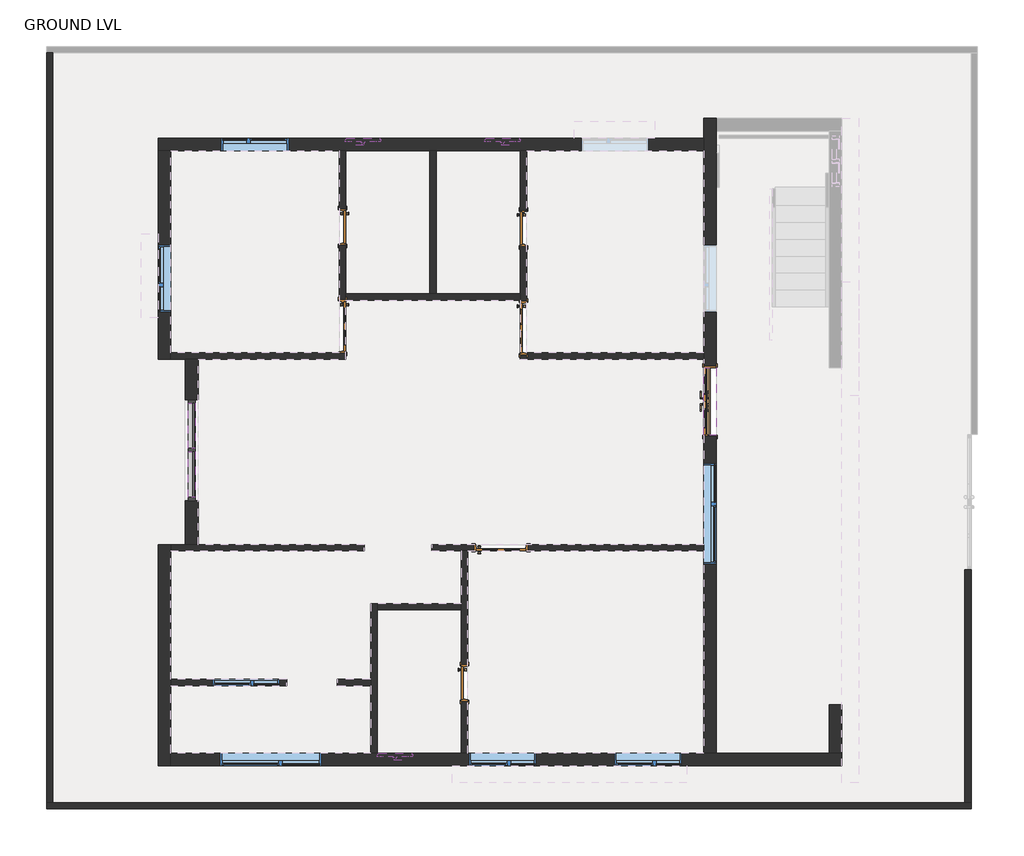
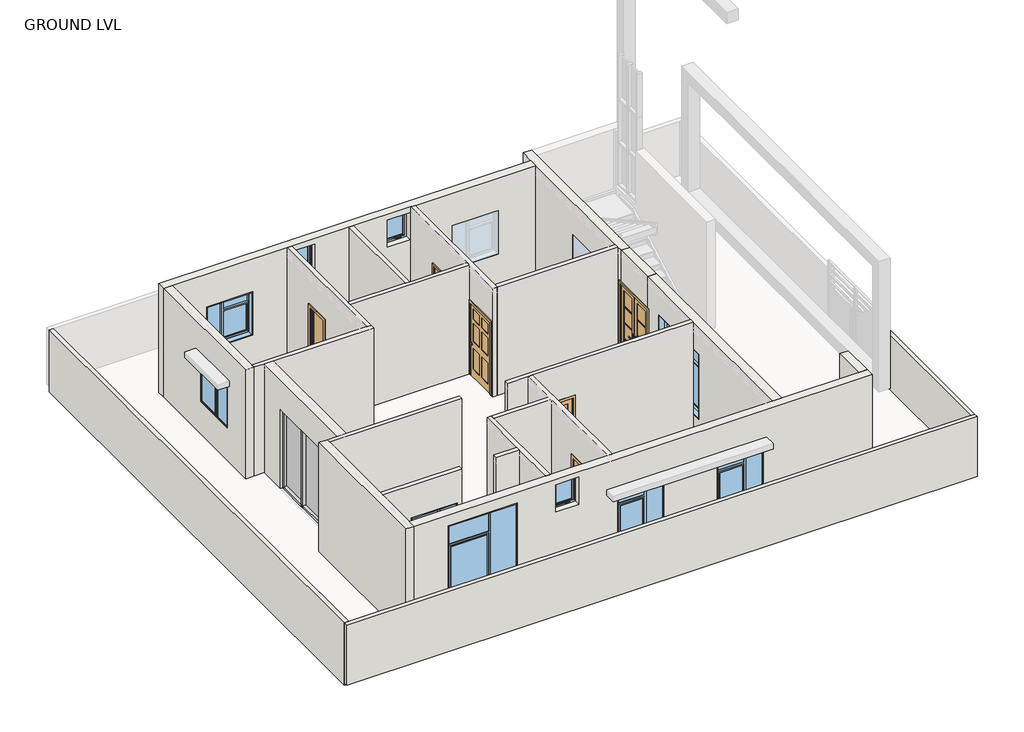
# One storey, part 1 of 2: 25 walls, 10 windows, 7 doors, 7 members, 2 plates.
"""IFC4 building model written with IfcOpenShell, lengths in millimetres."""

from ifc_helpers import new_model, si_unit, frame, origin, origin_with_axes, place, context, project, spatial, polyline, outline, extrude, faceted_brep, transform, mapped, element, save
from components import door_exterior_double_full_glass_wood_clad_double_main_door_4_3788f36b, door_92bad2d9, door_a4da38fb, door_0e119d28, door_525aa856, member_c17f1be2, member_acd63386, member_c841a703, system_panel_glazed_ef5431d1, window_610_x_762_5077743b, window_610_x_762_22856471, window_casement_double_sidelight_window_4_x_4_2a492e8f, window_casement_double_sidelight_window_4_x_4_ae1e99d1, window_casement_double_sidelight_window_6_x_6_6a7c62ef

model = new_model("IFC4")

# Units and contexts
model_context = context("Model", 3, world=origin())
ifc_project = project(units=[si_unit("LENGTHUNIT", "METRE", prefix="MILLI")], contexts=[model_context])

# Site, building, storey
site = spatial("IfcSite", under=ifc_project)
building = spatial("IfcBuilding", under=site)
storey = spatial("IfcBuildingStorey", under=building, Name="GROUND LVL", Elevation=0.0)

# Doors
placement = place(None, origin())
door_exterior_double_full_glass_wood_clad_double_main_door_4_shape = door_exterior_double_full_glass_wood_clad_double_main_door_4_3788f36b(model_context)
element("IfcDoor", 1, ObjectType="Door-Exterior-Double-Full Glass-Wood_Clad : double main door 4' x 7'", at=placement, inside=storey, context=model_context, shape_type="MappedRepresentation", body=[
    mapped(door_exterior_double_full_glass_wood_clad_double_main_door_4_shape, transform((-4646.5406154, 1972.1500875, -25.4), x_axis=(0.0, 1.0, 0.0), y_axis=(-1.0, 0.0, 0.0), z_axis=(0.0, 0.0, 1.0))),
])
door_shape = door_92bad2d9(model_context)
element("IfcDoor", 2, ObjectType="Door-Interior-Single-6_Panel-Wood : 36\" x 80\"", at=placement, inside=storey, context=model_context, shape_type="MappedRepresentation", body=[
    mapped(door_shape, transform((-11288.6406154, 3324.7000875, 0.0), x_axis=(0.0, -1.0, 0.0), y_axis=(1.0, 0.0, 0.0), z_axis=(0.0, 0.0, 1.0))),
])
door_2_shape = door_a4da38fb(model_context)
element("IfcDoor", 3, ObjectType="Door-Interior-Single-6_Panel-Wood : 36\" x 80\"", at=placement, inside=storey, context=model_context, shape_type="MappedRepresentation", body=[
    mapped(door_2_shape, transform((-8018.3906154, 3299.3000875, 0.0), x_axis=(0.0, -1.0, 0.0), y_axis=(1.0, 0.0, 0.0), z_axis=(0.0, 0.0, 1.0))),
])
element("IfcDoor", 4, ObjectType="Door-Interior-Single-6_Panel-Wood : 36\" x 80\"", at=placement, inside=storey, context=model_context, shape_type="MappedRepresentation", body=[
    mapped(door_2_shape, transform((-8421.6156154, -678.9749125, 0.0), x_axis=(1.0, 0.0, 0.0), y_axis=(0.0, 1.0, 0.0), z_axis=(0.0, 0.0, 1.0))),
])
door_3_shape = door_0e119d28(model_context)
element("IfcDoor", 5, ObjectType="Door-Interior-Single-Flush_Panel-Wood : 24\" x 80\"", at=placement, inside=storey, context=model_context, shape_type="MappedRepresentation", body=[
    mapped(door_3_shape, transform((-11288.6406154, 5128.1000875, 0.0), x_axis=(0.0, -1.0, 0.0), y_axis=(1.0, 0.0, 0.0), z_axis=(0.0, 0.0, 1.0))),
])
door_4_shape = door_525aa856(model_context)
element("IfcDoor", 6, ObjectType="Door-Interior-Single-Flush_Panel-Wood : 24\" x 80\"", at=placement, inside=storey, context=model_context, shape_type="MappedRepresentation", body=[
    mapped(door_4_shape, transform((-8018.3906154, 5102.7000875, 0.0), x_axis=(0.0, -1.0, 0.0), y_axis=(1.0, 0.0, 0.0), z_axis=(0.0, 0.0, 1.0))),
])
element("IfcDoor", 7, ObjectType="Door-Interior-Single-Flush_Panel-Wood : 24\" x 80\"", at=placement, inside=storey, context=model_context, shape_type="MappedRepresentation", body=[
    mapped(door_4_shape, transform((-9085.1906154, -3123.7249125, 0.0), x_axis=(0.0, -1.0, 0.0), y_axis=(1.0, 0.0, 0.0), z_axis=(0.0, 0.0, 1.0))),
])

# Members
member_shape = member_c17f1be2(model_context)
element("IfcMember", 8, ObjectType="Rectangular Mullion : 2.5\" x 5\" rectangular", at=placement, inside=storey, context=model_context, shape_type="MappedRepresentation", body=[
    mapped(member_shape, transform((-14015.9656154, 238.6000875, 2214.7649104), x_axis=(0.0, 0.0, 1.0), y_axis=(-1.0, 0.0, 0.0), z_axis=(0.0, -1.0, 0.0))),
])
element("IfcMember", 9, ObjectType="Rectangular Mullion : 2.5\" x 5\" rectangular", at=placement, inside=storey, context=model_context, shape_type="MappedRepresentation", body=[
    mapped(member_shape, transform((-14015.9656154, 1121.2500875, 2214.7649104), x_axis=(0.0, 0.0, 1.0), y_axis=(-1.0, 0.0, 0.0), z_axis=(0.0, -1.0, 0.0))),
])
element("IfcMember", 10, ObjectType="Rectangular Mullion : 2.5\" x 5\" rectangular", at=placement, inside=storey, context=model_context, shape_type="MappedRepresentation", body=[
    mapped(member_shape, transform((-14015.9656154, 1940.4000875, 0.0), x_axis=(0.0, 0.0, -1.0), y_axis=(-1.0, 0.0, 0.0), z_axis=(0.0, 1.0, 0.0))),
])
element("IfcMember", 11, ObjectType="Rectangular Mullion : 2.5\" x 5\" rectangular", at=placement, inside=storey, context=model_context, shape_type="MappedRepresentation", body=[
    mapped(member_shape, transform((-14015.9656154, 1057.7500875, 0.0), x_axis=(0.0, 0.0, -1.0), y_axis=(-1.0, 0.0, 0.0), z_axis=(0.0, 1.0, 0.0))),
])
member_2_shape = member_acd63386(model_context)
element("IfcMember", 12, ObjectType="Rectangular Mullion : 2.5\" x 5\" rectangular", at=placement, inside=storey, context=model_context, shape_type="MappedRepresentation", body=[
    mapped(member_2_shape, transform((-14015.9656154, 1089.5000875, 0.0), x_axis=(0.0, -1.0, 0.0), y_axis=(-1.0, 0.0, 0.0), z_axis=(0.0, 0.0, -1.0))),
])
member_3_shape = member_c841a703(model_context)
element("IfcMember", 13, ObjectType="Rectangular Mullion : 2.5\" x 5\" rectangular", at=placement, inside=storey, context=model_context, shape_type="MappedRepresentation", body=[
    mapped(member_3_shape, transform((-14015.9656154, 175.1000875, 0.0), x_axis=(0.0, -1.0, 0.0), y_axis=(-1.0, 0.0, 0.0), z_axis=(0.0, 0.0, -1.0))),
])
element("IfcMember", 14, ObjectType="Rectangular Mullion : 2.5\" x 5\" rectangular", at=placement, inside=storey, context=model_context, shape_type="MappedRepresentation", body=[
    mapped(member_3_shape, transform((-14015.9656154, 2003.9000875, 2214.7649104), x_axis=(0.0, 1.0, 0.0), y_axis=(-1.0, 0.0, 0.0), z_axis=(0.0, 0.0, 1.0))),
])

# Plates
system_panel_glazed_shape = system_panel_glazed_ef5431d1(model_context)
element("IfcPlate", 15, ObjectType="System Panel : Glazed", at=placement, inside=storey, context=model_context, shape_type="MappedRepresentation", body=[
    mapped(system_panel_glazed_shape, transform((-14015.9656154, 1530.8250875, 63.5), x_axis=(0.0, -1.0, 0.0), y_axis=(1.0, 0.0, 0.0), z_axis=(0.0, 0.0, 1.0))),
])
element("IfcPlate", 16, ObjectType="System Panel : Glazed", at=placement, inside=storey, context=model_context, shape_type="MappedRepresentation", body=[
    mapped(system_panel_glazed_shape, transform((-14015.9656154, 648.1750875, 63.5), x_axis=(0.0, -1.0, 0.0), y_axis=(1.0, 0.0, 0.0), z_axis=(0.0, 0.0, 1.0))),
])

# Walls
element("IfcWall", 17, at=placement, inside=storey, context=model_context, shape_type="Brep", body=[
    faceted_brep([(-4757.6656154, 6734.6500875, 0.0), (-14625.5656154, 6734.6500875, 0.0), (-14625.5656154, 6734.6500875, 3048.0), (-4757.6656154, 6734.6500875, 3048.0), (-10612.3656154, 6734.6500875, 2133.6), (-10612.3656154, 6734.6500875, 2895.6), (-11221.9656154, 6734.6500875, 2895.6), (-11221.9656154, 6734.6500875, 2133.6), (-8701.0156154, 6734.6500875, 2895.6), (-8701.0156154, 6734.6500875, 2133.6), (-8091.4156154, 6734.6500875, 2133.6), (-8091.4156154, 6734.6500875, 2895.6), (-5748.2656154, 6734.6500875, 2133.6), (-6967.4656154, 6734.6500875, 2133.6), (-6967.4656154, 6734.6500875, 914.4), (-5748.2656154, 6734.6500875, 914.4), (-12263.3656154, 6734.6500875, 2133.6), (-13482.5656154, 6734.6500875, 2133.6), (-13482.5656154, 6734.6500875, 914.4), (-12263.3656154, 6734.6500875, 914.4), (-4757.6656154, 6506.0500875, 0.0), (-4757.6656154, 6506.0500875, 3048.0), (-7958.0656154, 6506.0500875, 3048.0), (-8072.3656154, 6506.0500875, 3048.0), (-9596.3656154, 6506.0500875, 3048.0), (-9710.6656154, 6506.0500875, 3048.0), (-11234.6656154, 6506.0500875, 3048.0), (-11348.9656154, 6506.0500875, 3048.0), (-14396.9656154, 6506.0500875, 3048.0), (-14625.5656154, 6506.0500875, 3048.0), (-14625.5656154, 6506.0500875, 0.0), (-14396.9656154, 6506.0500875, 0.0), (-11348.9656154, 6506.0500875, 0.0), (-11234.6656154, 6506.0500875, 0.0), (-9710.6656154, 6506.0500875, 0.0), (-9596.3656154, 6506.0500875, 0.0), (-8072.3656154, 6506.0500875, 0.0), (-7958.0656154, 6506.0500875, 0.0), (-10612.3656154, 6506.0500875, 2895.6), (-10612.3656154, 6506.0500875, 2133.6), (-11221.9656154, 6506.0500875, 2133.6), (-11221.9656154, 6506.0500875, 2895.6), (-8701.0156154, 6506.0500875, 2133.6), (-8701.0156154, 6506.0500875, 2895.6), (-8091.4156154, 6506.0500875, 2895.6), (-8091.4156154, 6506.0500875, 2133.6), (-5748.2656154, 6506.0500875, 2133.6), (-5748.2656154, 6506.0500875, 914.4), (-6967.4656154, 6506.0500875, 914.4), (-6967.4656154, 6506.0500875, 2133.6), (-12263.3656154, 6506.0500875, 2133.6), (-12263.3656154, 6506.0500875, 914.4), (-13482.5656154, 6506.0500875, 914.4), (-13482.5656154, 6506.0500875, 2133.6)], [[[0, 1, 2, 3], [4, 5, 6, 7], [8, 9, 10, 11], [12, 13, 14, 15], [16, 17, 18, 19]], [[20, 21, 22, 23, 24, 25, 26, 27, 28, 29, 30, 31, 32, 33, 34, 35, 36, 37], [38, 39, 40, 41], [42, 43, 44, 45], [46, 47, 48, 49], [50, 51, 52, 53]], [[1, 0, 20, 37, 36, 35, 34, 33, 32, 31, 30]], [[3, 2, 29, 28, 27, 26, 25, 24, 23, 22, 21]], [[2, 1, 30, 29]], [[39, 38, 5, 4]], [[4, 7, 40, 39]], [[7, 6, 41, 40]], [[38, 41, 6, 5]], [[42, 9, 8, 43]], [[9, 42, 45, 10]], [[10, 45, 44, 11]], [[43, 8, 11, 44]], [[47, 46, 12, 15]], [[48, 47, 15, 14]], [[49, 48, 14, 13]], [[46, 49, 13, 12]], [[51, 50, 16, 19]], [[52, 51, 19, 18]], [[53, 52, 18, 17]], [[50, 53, 17, 16]], [[0, 3, 21, 20]]]),
])
element("IfcWall", 18, at=placement, inside=storey, context=model_context, shape_type="Brep", body=[
    faceted_brep([(-14625.5656154, 6506.0500875, 0.0), (-14625.5656154, 2734.1500875, 0.0), (-14625.5656154, 2734.1500875, 3048.0), (-14625.5656154, 6506.0500875, 3048.0), (-14625.5656154, 4803.1295492, 2133.6), (-14625.5656154, 3583.9295492, 2133.6), (-14625.5656154, 3583.9295492, 914.4), (-14625.5656154, 4803.1295492, 914.4), (-14396.9656154, 6506.0500875, 0.0), (-14396.9656154, 6506.0500875, 3048.0), (-14396.9656154, 2848.4500875, 3048.0), (-14396.9656154, 2734.1500875, 3048.0), (-14396.9656154, 2734.1500875, 0.0), (-14396.9656154, 2848.4500875, 0.0), (-14396.9656154, 4803.1295492, 2133.6), (-14396.9656154, 4803.1295492, 914.4), (-14396.9656154, 3583.9295492, 914.4), (-14396.9656154, 3583.9295492, 2133.6)], [[[0, 1, 2, 3], [4, 5, 6, 7]], [[8, 9, 10, 11, 12, 13], [14, 15, 16, 17]], [[1, 0, 8, 13, 12]], [[3, 2, 11, 10, 9]], [[0, 3, 9, 8]], [[2, 1, 12, 11]], [[15, 14, 4, 7]], [[16, 15, 7, 6]], [[17, 16, 6, 5]], [[14, 17, 5, 4]]]),
])
element("IfcWall", 19, at=placement, inside=storey, context=model_context, shape_type="Brep", body=[
    faceted_brep([(-14625.5656154, -618.6499125, 0.0), (-14625.5656154, -4619.1499125, 0.0), (-14625.5656154, -4619.1499125, 3048.0), (-14625.5656154, -618.6499125, 3048.0), (-14396.9656154, -618.6499125, 0.0), (-14396.9656154, -618.6499125, 3048.0), (-14396.9656154, -732.9499125, 3048.0), (-14396.9656154, -3057.0499125, 3048.0), (-14396.9656154, -3171.3499125, 3048.0), (-14396.9656154, -4390.5499125, 3048.0), (-14396.9656154, -4619.1499125, 3048.0), (-14396.9656154, -4619.1499125, 0.0), (-14396.9656154, -4390.5499125, 0.0), (-14396.9656154, -3171.3499125, 0.0), (-14396.9656154, -3057.0499125, 0.0), (-14396.9656154, -732.9499125, 0.0)], [[[0, 1, 2, 3]], [[4, 5, 6, 7, 8, 9, 10, 11, 12, 13, 14, 15]], [[1, 0, 4, 15, 14, 13, 12, 11]], [[3, 2, 10, 9, 8, 7, 6, 5]], [[2, 1, 11, 10]], [[0, 3, 5, 4]]]),
])
element("IfcWall", 20, at=placement, inside=storey, context=model_context, shape_type="Brep", body=[
    faceted_brep([(-14396.9656154, -4619.1499125, 0.0), (-2255.7656154, -4619.1499125, 0.0), (-2255.7656154, -4619.1499125, 3048.0), (-14396.9656154, -4619.1499125, 3048.0), (-10644.1156154, -4619.1499125, 2133.6), (-10644.1156154, -4619.1499125, 2895.6), (-10034.5156154, -4619.1499125, 2895.6), (-10034.5156154, -4619.1499125, 2133.6), (-9005.8156154, -4619.1499125, 2133.6), (-7786.6156154, -4619.1499125, 2133.6), (-7786.6156154, -4619.1499125, 914.4), (-9005.8156154, -4619.1499125, 914.4), (-6370.5656154, -4619.1499125, 2133.6), (-5151.3656154, -4619.1499125, 2133.6), (-5151.3656154, -4619.1499125, 914.4), (-6370.5656154, -4619.1499125, 914.4), (-13501.6156154, -4619.1499125, 2743.2), (-11672.8156154, -4619.1499125, 2743.2), (-11672.8156154, -4619.1499125, 914.4), (-13501.6156154, -4619.1499125, 914.4), (-14396.9656154, -4390.5499125, 0.0), (-14396.9656154, -4390.5499125, 3048.0), (-10777.4656154, -4390.5499125, 3048.0), (-10663.1656154, -4390.5499125, 3048.0), (-9139.1656154, -4390.5499125, 3048.0), (-9024.8656154, -4390.5499125, 3048.0), (-4757.6656154, -4390.5499125, 3048.0), (-4529.0656154, -4390.5499125, 3048.0), (-2484.3656154, -4390.5499125, 3048.0), (-2255.7656154, -4390.5499125, 3048.0), (-2255.7656154, -4390.5499125, 0.0), (-2484.3656154, -4390.5499125, 0.0), (-4529.0656154, -4390.5499125, 0.0), (-4757.6656154, -4390.5499125, 0.0), (-9024.8656154, -4390.5499125, 0.0), (-9139.1656154, -4390.5499125, 0.0), (-10663.1656154, -4390.5499125, 0.0), (-10777.4656154, -4390.5499125, 0.0), (-10644.1156154, -4390.5499125, 2895.6), (-10644.1156154, -4390.5499125, 2133.6), (-10034.5156154, -4390.5499125, 2133.6), (-10034.5156154, -4390.5499125, 2895.6), (-9005.8156154, -4390.5499125, 2133.6), (-9005.8156154, -4390.5499125, 914.4), (-7786.6156154, -4390.5499125, 914.4), (-7786.6156154, -4390.5499125, 2133.6), (-6370.5656154, -4390.5499125, 2133.6), (-6370.5656154, -4390.5499125, 914.4), (-5151.3656154, -4390.5499125, 914.4), (-5151.3656154, -4390.5499125, 2133.6), (-13501.6156154, -4390.5499125, 2743.2), (-13501.6156154, -4390.5499125, 914.4), (-11672.8156154, -4390.5499125, 914.4), (-11672.8156154, -4390.5499125, 2743.2)], [[[0, 1, 2, 3], [4, 5, 6, 7], [8, 9, 10, 11], [12, 13, 14, 15], [16, 17, 18, 19]], [[20, 21, 22, 23, 24, 25, 26, 27, 28, 29, 30, 31, 32, 33, 34, 35, 36, 37], [38, 39, 40, 41], [42, 43, 44, 45], [46, 47, 48, 49], [50, 51, 52, 53]], [[1, 0, 20, 37, 36, 35, 34, 33, 32, 31, 30]], [[3, 2, 29, 28, 27, 26, 25, 24, 23, 22, 21]], [[0, 3, 21, 20]], [[4, 39, 38, 5]], [[39, 4, 7, 40]], [[40, 7, 6, 41]], [[5, 38, 41, 6]], [[43, 42, 8, 11]], [[44, 43, 11, 10]], [[45, 44, 10, 9]], [[42, 45, 9, 8]], [[47, 46, 12, 15]], [[48, 47, 15, 14]], [[49, 48, 14, 13]], [[46, 49, 13, 12]], [[51, 50, 16, 19]], [[52, 51, 19, 18]], [[53, 52, 18, 17]], [[50, 53, 17, 16]], [[2, 1, 30, 29]]]),
])
element("IfcWall", 21, at=placement, inside=storey, context=model_context, shape_type="Brep", body=[
    faceted_brep([(-4529.0656154, 1362.5500875, 3048.0), (-4529.0656154, -4390.5499125, 3048.0), (-4529.0656154, -4390.5499125, 0.0), (-4529.0656154, 1337.1500875, 0.0), (-4529.0656154, 1337.1500875, 2133.6), (-4529.0656154, 1362.5500875, 2133.6), (-4529.0656154, -976.6434232, 2286.0), (-4529.0656154, 852.1565768, 2286.0), (-4529.0656154, 852.1565768, 457.2), (-4529.0656154, -976.6434232, 457.2), (-4757.6656154, -4390.5499125, 3048.0), (-4757.6656154, -732.9499125, 3048.0), (-4757.6656154, -618.6499125, 3048.0), (-4757.6656154, 1362.5500875, 3048.0), (-4757.6656154, 1362.5500875, 2133.6), (-4757.6656154, 1337.1500875, 2133.6), (-4757.6656154, 1337.1500875, 0.0), (-4757.6656154, -618.6499125, 0.0), (-4757.6656154, -732.9499125, 0.0), (-4757.6656154, -4390.5499125, 0.0), (-4757.6656154, -976.6434232, 2286.0), (-4757.6656154, -976.6434232, 457.2), (-4757.6656154, 852.1565768, 457.2), (-4757.6656154, 852.1565768, 2286.0)], [[[0, 1, 2, 3, 4, 5], [6, 7, 8, 9]], [[10, 11, 12, 13, 14, 15, 16, 17, 18, 19], [20, 21, 22, 23]], [[2, 19, 18, 17, 16, 3]], [[13, 0, 5, 14]], [[1, 0, 13, 12, 11, 10]], [[2, 1, 10, 19]], [[4, 15, 14, 5]], [[15, 4, 3, 16]], [[21, 20, 6, 9]], [[22, 21, 9, 8]], [[23, 22, 8, 7]], [[20, 23, 7, 6]]]),
])
element("IfcWall", 22, at=placement, inside=storey, context=model_context, shape_type="Brep", body=[
    faceted_brep([(-4529.0656154, 7090.2500875, 3048.0), (-4529.0656154, 6861.6500875, 3048.0), (-4529.0656154, 2581.7500875, 3048.0), (-4529.0656154, 2581.7500875, 2133.6), (-4529.0656154, 2607.1500875, 2133.6), (-4529.0656154, 2607.1500875, 0.0), (-4529.0656154, 6861.6500875, 0.0), (-4529.0656154, 7090.2500875, 0.0), (-4529.0656154, 4803.1295492, 2133.6), (-4529.0656154, 4803.1295492, 914.4), (-4529.0656154, 3583.9295492, 914.4), (-4529.0656154, 3583.9295492, 2133.6), (-4757.6656154, 2581.7500875, 3048.0), (-4757.6656154, 2734.1500875, 3048.0), (-4757.6656154, 2848.4500875, 3048.0), (-4757.6656154, 6506.0500875, 3048.0), (-4757.6656154, 6734.6500875, 3048.0), (-4757.6656154, 7090.2500875, 3048.0), (-4757.6656154, 7090.2500875, 0.0), (-4757.6656154, 6734.6500875, 0.0), (-4757.6656154, 6506.0500875, 0.0), (-4757.6656154, 2848.4500875, 0.0), (-4757.6656154, 2734.1500875, 0.0), (-4757.6656154, 2607.1500875, 0.0), (-4757.6656154, 2607.1500875, 2133.6), (-4757.6656154, 2581.7500875, 2133.6), (-4757.6656154, 4803.1295492, 2133.6), (-4757.6656154, 3583.9295492, 2133.6), (-4757.6656154, 3583.9295492, 914.4), (-4757.6656154, 4803.1295492, 914.4)], [[[0, 1, 2, 3, 4, 5, 6, 7], [8, 9, 10, 11]], [[12, 13, 14, 15, 16, 17, 18, 19, 20, 21, 22, 23, 24, 25], [26, 27, 28, 29]], [[18, 7, 6, 5, 23, 22, 21, 20, 19]], [[2, 1, 0, 17, 16, 15, 14, 13, 12]], [[2, 12, 25, 3]], [[4, 24, 23, 5]], [[24, 4, 3, 25]], [[9, 8, 26, 29]], [[10, 9, 29, 28]], [[11, 10, 28, 27]], [[8, 11, 27, 26]], [[0, 7, 18, 17]]]),
])
element("IfcWall", 23, at=placement, inside=storey, context=model_context, shape_type="Brep", body=[
    faceted_brep([(-14396.9656154, -732.9499125, 0.0), (-10895.4913348, -732.9499125, 0.0), (-10895.4913348, -732.9499125, 3048.0), (-14396.9656154, -732.9499125, 3048.0), (-14396.9656154, -618.6499125, 0.0), (-14396.9656154, -618.6499125, 3048.0), (-14130.2656154, -618.6499125, 3048.0), (-13901.6656154, -618.6499125, 3048.0), (-10895.4913348, -618.6499125, 3048.0), (-10895.4913348, -618.6499125, 0.0), (-13901.6656154, -618.6499125, 0.0), (-14130.2656154, -618.6499125, 0.0)], [[[0, 1, 2, 3]], [[4, 5, 6, 7, 8, 9, 10, 11]], [[1, 0, 4, 11, 10, 9]], [[2, 1, 9, 8]], [[3, 2, 8, 7, 6, 5]], [[0, 3, 5, 4]]]),
])
element("IfcWall", 24, at=placement, inside=storey, context=model_context, shape_type="SweptSolid", body=[
    extrude(outline(polyline([(0.0, -14396.9656154), (0.0, -12301.4656154), (3048.0, -12301.4656154), (3048.0, -14396.9656154), (0.0, -14396.9656154)]), holes=[polyline([(2133.6, -13647.6656154), (2133.6, -12428.4656154), (914.4, -12428.4656154), (914.4, -13647.6656154), (2133.6, -13647.6656154)])]), frame((0.0, -3171.3499125, 0.0), z_axis=(0.0, 1.0, 0.0), x_axis=(0.0, 0.0, 1.0)), (0.0, 0.0, 1.0), 114.3),
])
element("IfcWall", 25, at=placement, inside=storey, context=model_context, shape_type="SweptSolid", body=[
    extrude(outline(polyline([(-11387.0656154, -3057.0499125), (-10777.4656154, -3057.0499125), (-10777.4656154, -3171.3499125), (-11387.0656154, -3171.3499125), (-11387.0656154, -3057.0499125)])), origin_with_axes(), (0.0, 0.0, 1.0), 3048.0),
])
element("IfcWall", 26, at=placement, inside=storey, context=model_context, shape_type="Brep", body=[
    faceted_brep([(-10663.1656154, -4390.5499125, 0.0), (-10663.1656154, -1799.7499125, 0.0), (-10663.1656154, -1685.4499125, 0.0), (-10663.1656154, -1685.4499125, 3048.0), (-10663.1656154, -1799.7499125, 3048.0), (-10663.1656154, -4390.5499125, 3048.0), (-10777.4656154, -4390.5499125, 0.0), (-10777.4656154, -4390.5499125, 3048.0), (-10777.4656154, -3171.3499125, 3048.0), (-10777.4656154, -3057.0499125, 3048.0), (-10777.4656154, -1685.4499125, 3048.0), (-10777.4656154, -1685.4499125, 0.0), (-10777.4656154, -3057.0499125, 0.0), (-10777.4656154, -3171.3499125, 0.0)], [[[0, 1, 2, 3, 4, 5]], [[6, 7, 8, 9, 10, 11, 12, 13]], [[2, 1, 0, 6, 13, 12, 11]], [[5, 4, 3, 10, 9, 8, 7]], [[0, 5, 7, 6]], [[3, 2, 11, 10]]]),
])
element("IfcWall", 27, at=placement, inside=storey, context=model_context, shape_type="SweptSolid", body=[
    extrude(outline(polyline([(-9139.1656154, -1799.7499125), (-10663.1656154, -1799.7499125), (-10663.1656154, -1685.4499125), (-9139.1656154, -1685.4499125), (-9139.1656154, -1799.7499125)])), origin_with_axes(), (0.0, 0.0, 1.0), 3048.0),
])
element("IfcWall", 28, at=placement, inside=storey, context=model_context, shape_type="Brep", body=[
    faceted_brep([(-9024.8656154, -732.9499125, 3048.0), (-9024.8656154, -4390.5499125, 3048.0), (-9024.8656154, -4390.5499125, 0.0), (-9024.8656154, -3453.9249125, 0.0), (-9024.8656154, -3453.9249125, 2057.4), (-9024.8656154, -2793.5249125, 2057.4), (-9024.8656154, -2793.5249125, 0.0), (-9024.8656154, -732.9499125, 0.0), (-9139.1656154, -4390.5499125, 3048.0), (-9139.1656154, -1799.7499125, 3048.0), (-9139.1656154, -1685.4499125, 3048.0), (-9139.1656154, -732.9499125, 3048.0), (-9139.1656154, -732.9499125, 0.0), (-9139.1656154, -1685.4499125, 0.0), (-9139.1656154, -1799.7499125, 0.0), (-9139.1656154, -2793.5249125, 0.0), (-9139.1656154, -2793.5249125, 2057.4), (-9139.1656154, -3453.9249125, 2057.4), (-9139.1656154, -3453.9249125, 0.0), (-9139.1656154, -4390.5499125, 0.0)], [[[0, 1, 2, 3, 4, 5, 6, 7]], [[8, 9, 10, 11, 12, 13, 14, 15, 16, 17, 18, 19]], [[12, 7, 6, 15, 14, 13]], [[2, 19, 18, 3]], [[1, 0, 11, 10, 9, 8]], [[0, 7, 12, 11]], [[2, 1, 8, 19]], [[17, 4, 3, 18]], [[4, 17, 16, 5]], [[5, 16, 15, 6]]]),
])
element("IfcWall", 29, at=placement, inside=storey, context=model_context, shape_type="Brep", body=[
    faceted_brep([(-8072.3656154, 2734.1500875, 3048.0), (-8072.3656154, 3800.9500875, 3048.0), (-8072.3656154, 3915.2500875, 3048.0), (-8072.3656154, 6506.0500875, 3048.0), (-8072.3656154, 6506.0500875, 0.0), (-8072.3656154, 5432.9000875, 0.0), (-8072.3656154, 5432.9000875, 2057.4), (-8072.3656154, 4772.5000875, 2057.4), (-8072.3656154, 4772.5000875, 0.0), (-8072.3656154, 3915.2500875, 0.0), (-8072.3656154, 3800.9500875, 0.0), (-8072.3656154, 3781.9000875, 0.0), (-8072.3656154, 3781.9000875, 2057.4), (-8072.3656154, 2816.7000875, 2057.4), (-8072.3656154, 2816.7000875, 0.0), (-8072.3656154, 2734.1500875, 0.0), (-7958.0656154, 6506.0500875, 3048.0), (-7958.0656154, 2848.4500875, 3048.0), (-7958.0656154, 2734.1500875, 3048.0), (-7958.0656154, 2734.1500875, 0.0), (-7958.0656154, 2816.7000875, 0.0), (-7958.0656154, 2816.7000875, 2057.4), (-7958.0656154, 3781.9000875, 2057.4), (-7958.0656154, 3781.9000875, 0.0), (-7958.0656154, 4772.5000875, 0.0), (-7958.0656154, 4772.5000875, 2057.4), (-7958.0656154, 5432.9000875, 2057.4), (-7958.0656154, 5432.9000875, 0.0), (-7958.0656154, 6506.0500875, 0.0)], [[[0, 1, 2, 3, 4, 5, 6, 7, 8, 9, 10, 11, 12, 13, 14, 15]], [[16, 17, 18, 19, 20, 21, 22, 23, 24, 25, 26, 27, 28]], [[4, 28, 27, 5]], [[19, 15, 14, 20]], [[23, 11, 10, 9, 8, 24]], [[3, 2, 1, 0, 18, 17, 16]], [[4, 3, 16, 28]], [[0, 15, 19, 18]], [[14, 13, 21, 20]], [[13, 12, 22, 21]], [[12, 11, 23, 22]], [[7, 25, 24, 8]], [[25, 7, 6, 26]], [[26, 6, 5, 27]]]),
])
element("IfcWall", 30, at=placement, inside=storey, context=model_context, shape_type="Brep", body=[
    faceted_brep([(-8072.3656154, 3915.2500875, 0.0), (-9596.3656154, 3915.2500875, 0.0), (-9710.6656154, 3915.2500875, 0.0), (-11234.6656154, 3915.2500875, 0.0), (-11234.6656154, 3915.2500875, 3048.0), (-9710.6656154, 3915.2500875, 3048.0), (-9596.3656154, 3915.2500875, 3048.0), (-8072.3656154, 3915.2500875, 3048.0), (-8072.3656154, 3800.9500875, 0.0), (-8072.3656154, 3800.9500875, 3048.0), (-11234.6656154, 3800.9500875, 3048.0), (-11234.6656154, 3800.9500875, 0.0)], [[[0, 1, 2, 3, 4, 5, 6, 7]], [[8, 9, 10, 11]], [[3, 2, 1, 0, 8, 11]], [[7, 6, 5, 4, 10, 9]], [[0, 7, 9, 8]], [[4, 3, 11, 10]]]),
])
element("IfcWall", 31, at=placement, inside=storey, context=model_context, shape_type="Brep", body=[
    faceted_brep([(-11234.6656154, 6506.0500875, 3048.0), (-11234.6656154, 3915.2500875, 3048.0), (-11234.6656154, 3800.9500875, 3048.0), (-11234.6656154, 2848.4500875, 3048.0), (-11234.6656154, 2848.4500875, 2057.4), (-11234.6656154, 3807.3000875, 2057.4), (-11234.6656154, 3807.3000875, 0.0), (-11234.6656154, 3915.2500875, 0.0), (-11234.6656154, 4797.9000875, 0.0), (-11234.6656154, 4797.9000875, 2057.4), (-11234.6656154, 5458.3000875, 2057.4), (-11234.6656154, 5458.3000875, 0.0), (-11234.6656154, 6506.0500875, 0.0), (-11348.9656154, 2848.4500875, 3048.0), (-11348.9656154, 6506.0500875, 3048.0), (-11348.9656154, 6506.0500875, 0.0), (-11348.9656154, 5458.3000875, 0.0), (-11348.9656154, 5458.3000875, 2057.4), (-11348.9656154, 4797.9000875, 2057.4), (-11348.9656154, 4797.9000875, 0.0), (-11348.9656154, 3807.3000875, 0.0), (-11348.9656154, 3807.3000875, 2057.4), (-11348.9656154, 2848.4500875, 2057.4)], [[[0, 1, 2, 3, 4, 5, 6, 7, 8, 9, 10, 11, 12]], [[13, 14, 15, 16, 17, 18, 19, 20, 21, 22]], [[15, 12, 11, 16]], [[6, 20, 19, 8, 7]], [[3, 2, 1, 0, 14, 13]], [[0, 12, 15, 14]], [[3, 13, 22, 4]], [[21, 5, 4, 22]], [[5, 21, 20, 6]], [[18, 9, 8, 19]], [[9, 18, 17, 10]], [[10, 17, 16, 11]]]),
])
element("IfcWall", 32, at=placement, inside=storey, context=model_context, shape_type="SweptSolid", body=[
    extrude(outline(polyline([(-9710.6656154, 3915.2500875), (-9710.6656154, 6506.0500875), (-9596.3656154, 6506.0500875), (-9596.3656154, 3915.2500875), (-9710.6656154, 3915.2500875)])), origin_with_axes(), (0.0, 0.0, 1.0), 3048.0),
])
element("IfcWall", 33, at=placement, inside=storey, context=model_context, shape_type="Brep", body=[
    faceted_brep([(-14396.9656154, 2734.1500875, 0.0), (-14130.2656154, 2734.1500875, 0.0), (-13901.6656154, 2734.1500875, 0.0), (-11234.6656154, 2734.1500875, 0.0), (-11234.6656154, 2734.1500875, 3048.0), (-13901.6656154, 2734.1500875, 3048.0), (-14130.2656154, 2734.1500875, 3048.0), (-14396.9656154, 2734.1500875, 3048.0), (-14396.9656154, 2848.4500875, 3048.0), (-11348.9656154, 2848.4500875, 3048.0), (-11234.6656154, 2848.4500875, 3048.0), (-11234.6656154, 2848.4500875, 2057.4), (-11348.9656154, 2848.4500875, 2057.4), (-11348.9656154, 2848.4500875, 0.0), (-14396.9656154, 2848.4500875, 0.0), (-11348.9656154, 2842.1000875, 0.0), (-11234.6656154, 2842.1000875, 0.0), (-11234.6656154, 2842.1000875, 2057.4), (-11348.9656154, 2842.1000875, 2057.4)], [[[0, 1, 2, 3, 4, 5, 6, 7]], [[8, 9, 10, 11, 12, 13, 14]], [[3, 2, 1, 0, 14, 13, 15, 16]], [[7, 6, 5, 4, 10, 9, 8]], [[0, 7, 8, 14]], [[4, 3, 16, 17, 11, 10]], [[18, 15, 13, 12]], [[15, 18, 17, 16]], [[17, 18, 12, 11]]]),
])
element("IfcWall", 34, at=placement, inside=storey, context=model_context, shape_type="Brep", body=[
    faceted_brep([(-4757.6656154, 2848.4500875, 0.0), (-7958.0656154, 2848.4500875, 0.0), (-7958.0656154, 2848.4500875, 3048.0), (-4757.6656154, 2848.4500875, 3048.0), (-4757.6656154, 2734.1500875, 0.0), (-4757.6656154, 2734.1500875, 3048.0), (-7958.0656154, 2734.1500875, 3048.0), (-7958.0656154, 2734.1500875, 0.0), (-7958.0656154, 2816.7000875, 0.0)], [[[0, 1, 2, 3]], [[4, 5, 6, 7]], [[1, 0, 4, 7, 8]], [[3, 2, 6, 5]], [[2, 1, 8, 7, 6]], [[0, 3, 5, 4]]]),
])
element("IfcWall", 35, at=placement, inside=storey, context=model_context, shape_type="SweptSolid", body=[
    extrude(outline(polyline([(-4757.6656154, 1362.5500875), (-4757.6656154, 2581.7500875), (-4529.0656154, 2581.7500875), (-4529.0656154, 1362.5500875), (-4757.6656154, 1362.5500875)])), frame((0.0, 0.0, 2133.6), z_axis=(0.0, 0.0, 1.0), x_axis=(1.0, 0.0, 0.0)), (0.0, 0.0, 1.0), 914.4),
])
element("IfcWall", 36, at=placement, inside=storey, context=model_context, shape_type="Brep", body=[
    faceted_brep([(-9676.2913348, -618.6499125, 0.0), (-9676.2913348, -618.6499125, 3048.0), (-4757.6656154, -618.6499125, 3048.0), (-4757.6656154, -618.6499125, 0.0), (-7939.0156154, -618.6499125, 0.0), (-7939.0156154, -618.6499125, 2057.4), (-8904.2156154, -618.6499125, 2057.4), (-8904.2156154, -618.6499125, 0.0), (-9676.2913348, -732.9499125, 3048.0), (-9676.2913348, -732.9499125, 0.0), (-9139.1656154, -732.9499125, 0.0), (-9024.8656154, -732.9499125, 0.0), (-8904.2156154, -732.9499125, 0.0), (-8904.2156154, -732.9499125, 2057.4), (-7939.0156154, -732.9499125, 2057.4), (-7939.0156154, -732.9499125, 0.0), (-4757.6656154, -732.9499125, 0.0), (-4757.6656154, -732.9499125, 3048.0), (-9024.8656154, -732.9499125, 3048.0), (-9139.1656154, -732.9499125, 3048.0)], [[[0, 1, 2, 3, 4, 5, 6, 7]], [[8, 9, 10, 11, 12, 13, 14, 15, 16, 17, 18, 19]], [[9, 0, 7, 12, 11, 10]], [[3, 16, 15, 4]], [[1, 0, 9, 8]], [[2, 1, 8, 19, 18, 17]], [[3, 2, 17, 16]], [[14, 5, 4, 15]], [[5, 14, 13, 6]], [[6, 13, 12, 7]]]),
])
element("IfcWall", 37, at=placement, inside=storey, context=model_context, shape_type="SweptSolid", body=[
    extrude(outline(polyline([(-618.6499125, 3048.0), (2734.1500875, 3048.0), (2734.1500875, 0.0), (2003.9000875, 0.0), (2003.9000875, 2214.7649104), (175.1000875, 2214.7649104), (175.1000875, 0.0), (-618.6499125, 0.0), (-618.6499125, 3048.0)])), frame((-14130.2656154, 0.0, 0.0), z_axis=(1.0, 0.0, 0.0), x_axis=(0.0, 1.0, 0.0)), (0.0, 0.0, 1.0), 228.6),
])
element("IfcWall", 38, at=placement, inside=storey, context=model_context, shape_type="SweptSolid", body=[
    extrude(outline(polyline([(-2255.7656154, -3514.2499125), (-2255.7656154, -4390.5499125), (-2484.3656154, -4390.5499125), (-2484.3656154, -3514.2499125), (-2255.7656154, -3514.2499125)])), origin_with_axes(), (0.0, 0.0, 1.0), 3048.0),
])
element("IfcWall", 39, at=placement, inside=storey, context=model_context, shape_type="Brep", body=[
    faceted_brep([(82.5925412, -5287.2307263, -150.716329), (-16643.3074588, -5287.2307263, -150.716329), (-16643.3074588, -5287.2307263, 1524.0), (-16529.0074588, -5287.2307263, 1524.0), (-31.7074588, -5287.2307263, 1524.0), (82.5925412, -5287.2307263, 1524.0), (82.5925412, -5401.5307263, -150.716329), (82.5925412, -5401.5307263, 1524.0), (-16643.3074588, -5401.5307263, 1524.0), (-16643.3074588, -5401.5307263, -150.716329)], [[[0, 1, 2, 3, 4, 5]], [[6, 7, 8, 9]], [[1, 0, 6, 9]], [[5, 4, 3, 2, 8, 7]], [[2, 1, 9, 8]], [[0, 5, 7, 6]]]),
])
element("IfcWall", 40, at=placement, inside=storey, context=model_context, shape_type="Brep", body=[
    faceted_brep([(-16529.0074588, -5287.2307263, -218.1545864), (-16529.0074588, 8276.3692737, -218.1545864), (-16529.0074588, 8276.3692737, 1524.0), (-16529.0074588, -5287.2307263, 1524.0), (-16643.3074588, -5287.2307263, -218.1545864), (-16643.3074588, -5287.2307263, -150.716329), (-16643.3074588, -5287.2307263, 1524.0), (-16643.3074588, 8276.3692737, 1524.0), (-16643.3074588, 8276.3692737, -59.3518251), (-16643.3074588, 8276.3692737, -218.1545864)], [[[0, 1, 2, 3]], [[4, 5, 6, 7, 8, 9]], [[1, 0, 4, 9]], [[3, 2, 7, 6]], [[2, 1, 9, 8, 7]], [[0, 3, 6, 5, 4]]]),
])
element("IfcWall", 41, at=placement, inside=storey, context=model_context, shape_type="Brep", body=[
    faceted_brep([(82.5925412, -5287.2307263, -152.4), (82.5925412, -1077.1807263, -152.4), (82.5925412, -1077.1807263, 1524.0), (82.5925412, -5287.2307263, 1524.0), (82.5925412, -5287.2307263, -150.716329), (-31.7074588, -5287.2307263, -152.4), (-31.7074588, -5287.2307263, 1524.0), (-31.7074588, -1077.1807263, 1524.0), (-31.7074588, -1077.1807263, -152.4)], [[[0, 1, 2, 3, 4]], [[5, 6, 7, 8]], [[1, 0, 5, 8]], [[2, 1, 8, 7]], [[3, 2, 7, 6]], [[0, 4, 3, 6, 5]]]),
])

# Windows
window_610_x_762_shape = window_610_x_762_5077743b(model_context)
element("IfcWindow", 42, ObjectType="610 x 762", at=placement, inside=storey, context=model_context, shape_type="MappedRepresentation", body=[
    mapped(window_610_x_762_shape, transform((-10917.1656154, 6620.3500875, 1333.6), x_axis=(-1.0, 0.0, 0.0), y_axis=(0.0, -1.0, 0.0), z_axis=(0.0, 0.0, 1.0))),
])
window_610_x_762_2_shape = window_610_x_762_22856471(model_context)
element("IfcWindow", 43, ObjectType="610 x 762", at=placement, inside=storey, context=model_context, shape_type="MappedRepresentation", body=[
    mapped(window_610_x_762_2_shape, transform((-8396.2156154, 6620.3500875, 1333.6), x_axis=(1.0, 0.0, 0.0), y_axis=(0.0, 1.0, 0.0), z_axis=(0.0, 0.0, 1.0))),
])
element("IfcWindow", 44, ObjectType="610 x 762", at=placement, inside=storey, context=model_context, shape_type="MappedRepresentation", body=[
    mapped(window_610_x_762_2_shape, transform((-10339.3156154, -4504.8499125, 1333.6), x_axis=(1.0, 0.0, 0.0), y_axis=(0.0, 1.0, 0.0), z_axis=(0.0, 0.0, 1.0))),
])
window_casement_double_sidelight_window_4_x_4_shape = window_casement_double_sidelight_window_4_x_4_2a492e8f(model_context)
element("IfcWindow", 45, ObjectType="Window-Casement-Double-Sidelight : window 4' x 4'", at=placement, inside=storey, context=model_context, shape_type="MappedRepresentation", body=[
    mapped(window_casement_double_sidelight_window_4_x_4_shape, transform((-8396.2156154, -4504.8499125, 0.0), x_axis=(-1.0, 0.0, 0.0), y_axis=(0.0, -1.0, 0.0), z_axis=(0.0, 0.0, 1.0))),
])
element("IfcWindow", 46, ObjectType="Window-Casement-Double-Sidelight : window 4' x 4'", at=placement, inside=storey, context=model_context, shape_type="MappedRepresentation", body=[
    mapped(window_casement_double_sidelight_window_4_x_4_shape, transform((-5760.9656154, -4504.8499125, 0.0), x_axis=(-1.0, 0.0, 0.0), y_axis=(0.0, -1.0, 0.0), z_axis=(0.0, 0.0, 1.0))),
])
element("IfcWindow", 47, ObjectType="Window-Casement-Double-Sidelight : window 4' x 4'", at=placement, inside=storey, context=model_context, shape_type="MappedRepresentation", body=[
    mapped(window_casement_double_sidelight_window_4_x_4_shape, transform((-12872.9656154, 6620.3500875, 0.0), x_axis=(1.0, 0.0, 0.0), y_axis=(0.0, 1.0, 0.0), z_axis=(0.0, 0.0, 1.0))),
])
element("IfcWindow", 48, ObjectType="Window-Casement-Double-Sidelight : window 4' x 4'", at=placement, inside=storey, context=model_context, shape_type="MappedRepresentation", body=[
    mapped(window_casement_double_sidelight_window_4_x_4_shape, transform((-14511.2656154, 4193.5295492, 0.0), x_axis=(0.0, 1.0, 0.0), y_axis=(-1.0, 0.0, 0.0), z_axis=(0.0, 0.0, 1.0))),
])
window_casement_double_sidelight_window_4_x_4_2_shape = window_casement_double_sidelight_window_4_x_4_ae1e99d1(model_context)
element("IfcWindow", 49, ObjectType="Window-Casement-Double-Sidelight : window 4' x 4'", at=placement, inside=storey, context=model_context, shape_type="MappedRepresentation", body=[
    mapped(window_casement_double_sidelight_window_4_x_4_2_shape, transform((-13038.0656154, -3114.1999125, 0.0), x_axis=(-1.0, 0.0, 0.0), y_axis=(0.0, -1.0, 0.0), z_axis=(0.0, 0.0, 1.0))),
])
window_casement_double_sidelight_window_6_x_6_shape = window_casement_double_sidelight_window_6_x_6_6a7c62ef(model_context)
element("IfcWindow", 50, ObjectType="Window-Casement-Double-Sidelight : window 6' x 6'", at=placement, inside=storey, context=model_context, shape_type="MappedRepresentation", body=[
    mapped(window_casement_double_sidelight_window_6_x_6_shape, transform((-12587.2156154, -4504.8499125, 0.0), x_axis=(-1.0, 0.0, 0.0), y_axis=(0.0, -1.0, 0.0), z_axis=(0.0, 0.0, 1.0))),
])
element("IfcWindow", 51, ObjectType="Window-Casement-Double-Sidelight : window 6' x 6'", at=placement, inside=storey, context=model_context, shape_type="MappedRepresentation", body=[
    mapped(window_casement_double_sidelight_window_6_x_6_shape, transform((-4643.3656154, -62.2434232, -457.2), x_axis=(0.0, -1.0, 0.0), y_axis=(1.0, 0.0, 0.0), z_axis=(0.0, 0.0, 1.0))),
])

save(model, "model.ifc")

# Revit data of these elements
# Type "Door-Exterior-Double-Full Glass-Wood_Clad : double main door 4' x 7'"
#   Type Mark = "14"
#   Assembly Code = "B2030100"
#   Analytic Construction = "French door, wood frame with double glass"
#   Top Rail = 0' - 4 11/16"
#   Threshold Offset [instance default] = 0' - 0 1/2"
#   Thickness = 0' - 1 3/8"
#   Thermal Resistance (R) = 1.9158 (h·ft²·°F)/BTU
#   Swing Angle [instance default] = 90.00°
#   Stiles = 0' - 4 3/4"
#   Rough Width = 4' - 2"
#   Rough Height = 7' - 1"
#   Panel Width = 2' - 0"
#   Door Offset [instance default] = 0' - 0"
#   Height = 7' - 0"
#   Width = 4' - 0"
#   Heat Transfer Coefficient (U) = 0.5220 BTU/(h·ft²·°F)
#   Bottom Rail = 0' - 9 1/8"
#   Exterior Trim [instance default] = yes
#   Threshold [instance default] = yes
#   Show Grill [instance default] = yes
#   Function = 1
#   Trim Material = Cherry
#   Threshold Material = Cherry
#   Panel Material = Cherry
#   Glazing = Glass
#   Frame Material = Cherry
#   Door Handle Material = Aluminum
#   Visual Light Transmittance = 0
#   Solar Heat Gain Coefficient = 0
#   Wall Closure = (empty or 0)
#   Construction Type = (empty or 0)
# Type "Door-Interior-Single-6_Panel-Wood : 36\" x 80\""
#   Type Mark = "9"
#   Assembly Code = "C1020300"
#   Analytic Construction = "Wooden"
#   Top Rail = 0' - 4 11/16"
#   Top Panel = 0' - 11"
#   Thickness = 0' - 1 3/8"
#   Thermal Resistance (R) = 2.5876 (h·ft²·°F)/BTU
#   Swing Angle [instance default] = 90.00°
#   Stiles = 0' - 4 3/4"
#   Rough Width = 3' - 2"
#   Rough Height = 6' - 9"
#   Mullion = 0' - 4 1/2"
#   Lock Rail = 0' - 7 1/2"
#   Intermediate Rail = 0' - 4 1/2"
#   Height = 6' - 8"
#   Width = 3' - 0"
#   Heat Transfer Coefficient (U) = 0.3865 BTU/(h·ft²·°F)
#   Bottom Rail = 0' - 9 1/8"
#   Trim Material = Cherry
#   Panel Material = Cherry
#   Frame Material = Cherry
#   Door Handle Material = Aluminum
#   Visual Light Transmittance = 0
#   Solar Heat Gain Coefficient = 0
#   Wall Closure = (empty or 0)
#   Function = (empty or 0)
# Type "Door-Interior-Single-Flush_Panel-Wood : 24\" x 80\""
#   Type Mark = "12"
#   Assembly Code = "C1020300"
#   Analytic Construction = "Wooden"
#   Thickness = 0' - 1 3/8"
#   Thermal Resistance (R) = 2.5876 (h·ft²·°F)/BTU
#   Swing Angle [instance default] = 90.00°
#   Rough Width = 2' - 2"
#   Rough Height = 6' - 9"
#   Height = 6' - 8"
#   Width = 2' - 0"
#   Heat Transfer Coefficient (U) = 0.3865 BTU/(h·ft²·°F)
#   Trim Material = Cherry
#   Panel Material = Cherry
#   Frame Material = Cherry
#   Door Handle Material = Aluminum
#   Visual Light Transmittance = 0
#   Solar Heat Gain Coefficient = 0
#   Wall Closure = (empty or 0)
#   Function = (empty or 0)
# Type "Rectangular Mullion : 2.5\" x 5\" rectangular"
#   built-in parameter 1007304 = 0.416667 (stored number, unit not read)
#   built-in parameter 1007301 = 0.104167 (stored number, unit not read)
#   built-in parameter 1007300 = 0.104167 (stored number, unit not read)
# Type "System Panel : Glazed"
#   Construction Type Id = "GSP4R"
#   Analytic Construction = "1/8 in Pilkington single glazing"
#   Visual Light Transmittance = 0.9
#   Solar Heat Gain Coefficient = 0.86
#   Heat Transfer Coefficient (U) = 1.18115 BTU/(h·ft²·°F)
#   Define Thermal Properties by = 1
# Type
#   Assembly Code = "B2010"
#   Layers, outside or top first: 0' - 9" "LIGHT BEIGE" (function 1)
# Type
#   Assembly Code = "B2010"
#   Layers, outside or top first: 0' - 4 1/2" "LIGHT BEIGE" (function 1)
# Type "610 x 762"
#   Type Mark = "18"
#   Water resistance = "up to Class E1050, PN-EN 12208:2001"
#   URL = "https://aluprof.com/en/architects/offer/window-and-door-systems/mb-59s-casement-mb-59s-casement-hi"
#   Type IFC Predefined Type = "NOTDEFINED"
#   Resistance to wind load = "up to Class C5, PN-EN 12210:2016"
#   Operation = "SingleTopHungCasement"
#   Opening type = "Top-hung casement opening outwards"
#   Model = "MB-59S Casement"
#   ManufacturerSustainabilityPolicyURL = "https://aluprof.eu/en/company/sustainable-development"
#   Manufacturer = "ALUPROF SA"
#   Keynote = "08511300"
#   IfcExportType = "NOTDEFINED"
#   IfcExportAs = "IfcWindowType"
#   Hardware [instance default] = ""
#   Handle type [instance default] = ""
#   Glazing construction = "4/16/4"
#   Export Type to IFC As = "IfcWindowType"
#   Description = "Single top-hung casement opening outwards"
#   Content of the recyclate in the material = "69.2%"
#   COBie.Type.Name = "MB-59S Casement"
#   COBie.Type.Manufacturer = "ALUPROF SA\r\nALUPROF S.A.\r\nALUPROF S.A."
#   Assembly Code = "B2020110"
#   Analytic Construction = "<None>"
#   Air permeability = "up to Class 4, PN-EN 12207:2001"
#   Thermal insulation = 0.299387 BTU/(h·ft²·°F)
#   Sash thickness = 0' - 2.32283"
#   Rough Width = 2' - 1.1811"
#   Rough Height = 2' - 7.1811"
#   Reference line height [instance default] = 0' - 0"
#   Opening angle [instance default] = 0.00°
#   Mounting space = 0' - 0.59055"
#   Height = 2' - 6"
#   Glazing area = 2.82349 SF
#   Frame thickness = 0' - 1.9685"
#   Exterior wall face offset = 0' - 0.7874"
#   Sill Height = 2' - 7.49606"
#   Width = 2' - 0"
#   Warm installation [instance default] = yes
#   Thermal variant HI = no
#   Schedule No. [instance default] = 1
#   IsWindowOpen [instance default] = no
#   IsExternal = yes
#   Define Thermal Properties by = 1
#   COBie.Type = yes
#   COBie = yes
#   Wall Closure = (empty or 0)
# Type "Window-Casement-Double-Sidelight : window 4' x 4'"
#   Type Mark = "22"
#   Fire Rating = "0.5h"
#   Assembly Code = "B2020100"
#   Analytic Construction = "Double glazing - domestic"
#   Window Inset [instance default] = 0' - 0 5/8"
#   Wall Thickness [instance default] = 0' - 6"
#   Visual Light Transmittance = 0.81
#   Transom Height Ratio = 0.3
#   Transom Height = 1' - 2.4"
#   Thermal Resistance (R) = 1.8146 (h·ft²·°F)/BTU
#   Solar Heat Gain Coefficient = 0.76
#   Side Width = 1' - 7.2"
#   Rough Width = 4' - 0 1/2"
#   Rough Height = 4' - 0 1/2"
#   Opening Window Width = 2' - 4.8"
#   Opening Window Height = 2' - 9.6"
#   Heat Transfer Coefficient (U) = 0.5511 BTU/(h·ft²·°F)
#   Height = 4' - 0"
#   Frame Gap 3 [instance default] = 0' - 1 83/128"
#   Frame Gap 2 [instance default] = 0' - 0 5/8"
#   Frame Gap 1 = 0' - 1 51/128"
#   Default Sill Height = 3' - 0"
#   Width = 4' - 0"
#   Frame Material = Metal - Aluminum
#   Glass Panel Material = Glass
#   Wall Closure = (empty or 0)
# Type "Window-Casement-Double-Sidelight : window 6' x 6'"
#   Type Mark = "23"
#   Fire Rating = "0.5h"
#   Assembly Code = "B2020100"
#   Analytic Construction = "Double glazing - domestic"
#   Window Inset [instance default] = 0' - 0 5/8"
#   Wall Thickness [instance default] = 0' - 6"
#   Visual Light Transmittance = 0.81
#   Transom Height Ratio = 0.3
#   Transom Height = 1' - 9.6"
#   Thermal Resistance (R) = 1.8146 (h·ft²·°F)/BTU
#   Solar Heat Gain Coefficient = 0.76
#   Side Width = 2' - 4.8"
#   Rough Width = 6' - 0 1/2"
#   Rough Height = 6' - 0 1/2"
#   Opening Window Width = 3' - 7.2"
#   Opening Window Height = 4' - 2.4"
#   Heat Transfer Coefficient (U) = 0.5511 BTU/(h·ft²·°F)
#   Height = 6' - 0"
#   Frame Gap 3 [instance default] = 0' - 1 83/128"
#   Frame Gap 2 [instance default] = 0' - 0 5/8"
#   Frame Gap 1 = 0' - 1 51/128"
#   Default Sill Height = 3' - 0"
#   Width = 6' - 0"
#   Frame Material = Metal - Aluminum
#   Glass Panel Material = Glass
#   Wall Closure = (empty or 0)
# Element 1 (IfcDoor, "Door-Exterior-Double-Full Glass-Wood_Clad : double main door 4' x 7'")
#   Threshold Offset = 0' - 0 1/2"
#   Swing Angle = 90.00°
#   Door Offset = 0' - 0"
#   Threshold = yes
#   Show Grill = yes
#   Exterior Trim = yes
#   Phase Created = New Construction
#   Materials on its faces: "Cherry", "Aluminum", "Glass"
# Elements 2, 3, 4 (IfcDoor, "Door-Interior-Single-6_Panel-Wood : 36\" x 80\"")
#   Swing Angle = 90.00°
#   Phase Created = New Construction
#   Materials on its faces: "Cherry", "Aluminum"
# Elements 5, 6, 7 (IfcDoor, "Door-Interior-Single-Flush_Panel-Wood : 24\" x 80\"")
#   Swing Angle = 90.00°
#   Phase Created = New Construction
#   Materials on its faces: "Cherry", "Aluminum"
# Elements 8, 9, 10, 11, 12, 13, 14 (IfcMember, "Rectangular Mullion : 2.5\" x 5\" rectangular")
#   Phase Created = New Construction
#   Materials on its faces: "Aluminum"
# Elements 15, 16 (IfcPlate, "System Panel : Glazed")
#   Phase Created = New Construction
#   Materials on its faces: "Glass"
# Elements 17, 18, 19, 21, 22, 23, 24, 25, 26, 27, 28, 29, 30, 31, 32, 33, 34, 35, 36, 37 (IfcWall)
#   Top Offset = 0' - 0"
#   Base Offset = 0' - 0"
#   wall height = 10' - 0"
#   Phase Created = New Construction
#   Base Constraint = GROUND LVL
#   Top Constraint = FIRST FLOOR
#   Materials on its faces: "LIGHT BEIGE"
# Elements 20, 38 (IfcWall)
#   Top Offset = 0' - 0"
#   Base Offset = 0' - 0"
#   wall height = 10' - 0"
#   Phase Created = New Construction
#   Base Constraint = GROUND LVL
#   Top Constraint = FIRST FLOOR
#   Materials on its faces: "LIGHT BEIGE", "Concrete, Cast-in-Place gray"
# Element 39 (IfcWall)
#   built-in parameter 1001111 = -0' - 5.93371"
#   Top Offset = 0' - 0"
#   Base Offset = -0' - 5.93371"
#   Unconnected Height = 5' - 5.93371"
#   wall height = 5' - 5.93371"
#   Phase Created = New Construction
#   Base Constraint = GROUND LVL
#   Materials on its faces: "LIGHT BEIGE"
# Element 40 (IfcWall)
#   built-in parameter 1001111 = -0' - 8.58876"
#   Top Offset = 0' - 0"
#   Base Offset = -0' - 8.58876"
#   Unconnected Height = 5' - 8.58876"
#   wall height = 5' - 8.58876"
#   Phase Created = New Construction
#   Base Constraint = GROUND LVL
#   Materials on its faces: "LIGHT BEIGE"
# Element 41 (IfcWall)
#   built-in parameter 1001111 = -0' - 6"
#   Top Offset = 0' - 0"
#   Base Offset = -0' - 6"
#   Unconnected Height = 5' - 6"
#   wall height = 5' - 6"
#   Phase Created = New Construction
#   Base Constraint = GROUND LVL
#   Materials on its faces: "LIGHT BEIGE"
# Element 42 (IfcWindow, "610 x 762")
#   Mark = "1"
#   Hardware = ""
#   Handle type = ""
#   Reference line height = 0' - 0"
#   Opening angle = 0.00°
#   Warm installation = yes
#   Schedule No. = 1
#   IsWindowOpen = no
#   Phase Created = New Construction
# Element 43 (IfcWindow, "610 x 762")
#   Mark = "2"
#   Hardware = ""
#   Handle type = ""
#   Reference line height = 0' - 0"
#   Opening angle = 0.00°
#   Warm installation = yes
#   Schedule No. = 1
#   IsWindowOpen = no
#   Phase Created = New Construction
# Element 44 (IfcWindow, "610 x 762")
#   Mark = "3"
#   Hardware = ""
#   Handle type = ""
#   Reference line height = 0' - 0"
#   Opening angle = 0.00°
#   Warm installation = yes
#   Schedule No. = 1
#   IsWindowOpen = no
#   Phase Created = New Construction
# Element 45 (IfcWindow, "Window-Casement-Double-Sidelight : window 4' x 4'")
#   Mark = "4"
#   Window Inset = 0' - 0 5/8"
#   Frame Gap 3 = 0' - 1 83/128"
#   Frame Gap 2 = 0' - 0 5/8"
#   Phase Created = New Construction
#   Materials on its faces: "Metal - Aluminum", "Glass"
# Element 46 (IfcWindow, "Window-Casement-Double-Sidelight : window 4' x 4'")
#   Mark = "5"
#   Window Inset = 0' - 0 5/8"
#   Frame Gap 3 = 0' - 1 83/128"
#   Frame Gap 2 = 0' - 0 5/8"
#   Phase Created = New Construction
#   Materials on its faces: "Metal - Aluminum", "Glass"
# Element 47 (IfcWindow, "Window-Casement-Double-Sidelight : window 4' x 4'")
#   Mark = "11"
#   Window Inset = 0' - 0 5/8"
#   Frame Gap 3 = 0' - 1 83/128"
#   Frame Gap 2 = 0' - 0 5/8"
#   Phase Created = New Construction
#   Materials on its faces: "Metal - Aluminum", "Glass"
# Element 48 (IfcWindow, "Window-Casement-Double-Sidelight : window 4' x 4'")
#   Mark = "12"
#   Window Inset = 0' - 0 5/8"
#   Frame Gap 3 = 0' - 1 83/128"
#   Frame Gap 2 = 0' - 0 5/8"
#   Phase Created = New Construction
#   Materials on its faces: "Metal - Aluminum", "Glass"
# Element 49 (IfcWindow, "Window-Casement-Double-Sidelight : window 4' x 4'")
#   Mark = "7"
#   Window Inset = 0' - 0 5/8"
#   Frame Gap 3 = 0' - 1 83/128"
#   Frame Gap 2 = 0' - 0 5/8"
#   Phase Created = New Construction
#   Materials on its faces: "Metal - Aluminum", "Glass"
# Element 50 (IfcWindow, "Window-Casement-Double-Sidelight : window 6' x 6'")
#   Mark = "6"
#   Window Inset = 0' - 0 5/8"
#   Frame Gap 3 = 0' - 1 83/128"
#   Frame Gap 2 = 0' - 0 5/8"
#   Phase Created = New Construction
#   Materials on its faces: "Metal - Aluminum", "Glass"
# Element 51 (IfcWindow, "Window-Casement-Double-Sidelight : window 6' x 6'")
#   Mark = "9"
#   Window Inset = 0' - 0 5/8"
#   Frame Gap 3 = 0' - 1 83/128"
#   Frame Gap 2 = 0' - 0 5/8"
#   Phase Created = New Construction
#   Materials on its faces: "Metal - Aluminum", "Glass"
# Materials
#   "Cherry": class "Wood", colour RGB 226 177 128, transparency 0, Description = "Prunus Serotina", Cost = 0
#   "Glass": class "Glass", colour RGB 0 128 192, transparency 0.75, Description = "Soda Lime Glass", Cost = 0
#   "Aluminum": class "Metal", colour RGB 247 247 247, transparency 0, Description = "Aluminum 6061", Cost = 0
#   "LIGHT BEIGE": class "Generic", colour RGB 120 120 120, transparency 0, Cost = 0
#   "Metal - Aluminum": class "Metal", colour RGB 247 247 247, transparency 0
#   "Concrete, Cast-in-Place gray": class "Concrete", colour RGB 192 192 192, transparency 0, Description = "Cast-in-place concrete", Cost = 0
